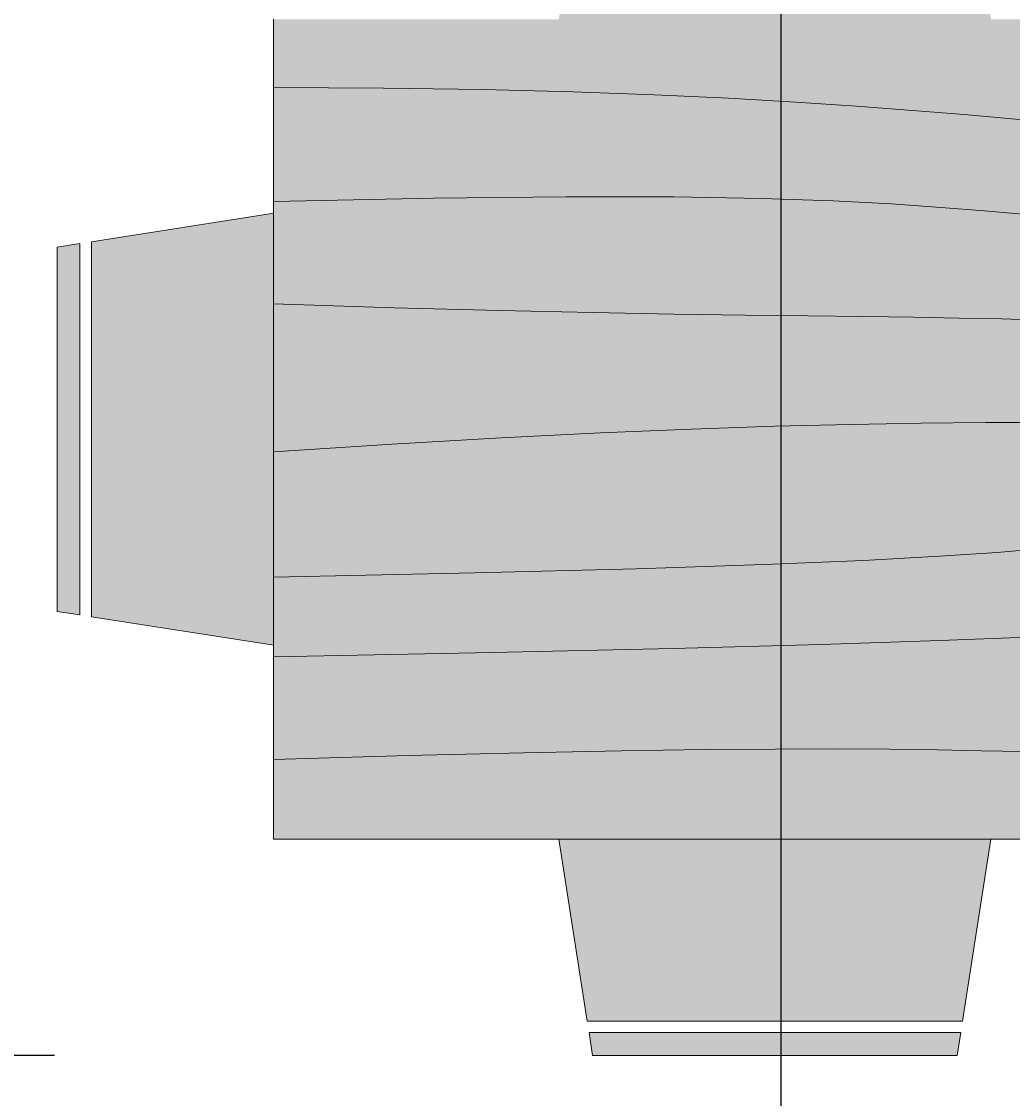
# Model space of a CAD drawing. Units: inches. Extents: x 2549 to 3108, y 1683 to 2362.
# Tile 9 of 30: x 2711 to 2734, y 2016 to 2041. Entities that reach past the tile are written whole.
import ezdxf

# ---------------------------------------------------------------- set-up
doc = ezdxf.new("R2010")
doc.units = ezdxf.units.IN
for name, color, linetype, lineweight in [('A-ANNO-DIMS', 2, 'Continuous', 18), ('A-FURN', 8, 'Continuous', 18), ('A-FURN-PATT', 9, 'Continuous', 13)]:
    doc.layers.add(name, color=color, linetype=linetype, lineweight=lineweight)
doc.layers.add('C-PKNG-VEHI-PATT', color=251, linetype='Continuous', lineweight=13, true_color=0x636466)
doc.layers.add('C-PVMT-PATT', color=9, linetype='Continuous', lineweight=13, true_color=0xc7c8ca)
doc.styles.get("Standard").update_dxf_attribs({"font": 'arial.ttf'})
doc.dimstyles.get("Standard").update_dxf_attribs({"dimtxt": 0.18, "dimasz": 0.18, "dimexe": 0.18, "dimexo": 0.0625, "dimgap": 0.09, "dimtad": 0, "dimtih": 1, "dimtoh": 1, "dimdec": 4, "dimzin": 0, "dimdsep": 46, "dimtxsty": 'Standard', "dimcen": 0.09, "dimadec": 0, "dimazin": 0, "dimtfac": 1, "dimtdec": 4, "dimtofl": 0, "dimtmove": 0, "dimatfit": 3, "dimfxl": 1, "dimtolj": 1, "dimtzin": 0, "dimarcsym": 0})

# ---------------------------------------------------------------- blocks, each defined once
blk = doc.blocks.new('Dining Set - 36 x 72 in.')
for p, q in [((-36, 18), (-36, -18)), ((-44.0006, 8.23428), (-35.9976, 9.48474)), ((-45.5, 8), (-44.5004, 8.15617)), ((-44.5, -8.15843), (-44.5, 8.15338)), ((-44, 8.23041), (-44, -8.23915)), ((-45.5, 8), (-45.5, -8)), ((-44.4997, -8.15631), (-45.5, -8)), ((-35.9976, -9.48476), (-43.9993, -8.2345)), ((-36, -18), (36, -18)), ((-22.2343, -26.0006), (-23.4847, -17.99762)), ((-4.5152, -17.99762), (-5.7655, -25.99928)), ((-22.2304, -26), (-5.7608, -26)), ((-22, -27.5), (-22.1562, -26.50044)), ((-5.8416, -26.5), (-22.1534, -26.5)), ((-5.8437, -26.49967), (-6, -27.5)), ((-22, -27.5), (-6, -27.5))]:
    blk.add_line(p, q)
for points in [[(-36, 15), (-31.1772, 14.97754), (-26.8079, 14.91406), (-22.8538, 14.81543), (-19.276, 14.6875), (-16.0362, 14.53613), (-13.0957, 14.36718), (-10.4159, 14.18652), (-7.9583, 14), (-5.6904, 13.81315), (-3.6035, 13.63021), (-1.6954, 13.45508)], [(-36, 10), (-28.9766, 10.14274), (-23.1725, 10.20442), (-18.4241, 10.19775), (-14.5677, 10.13541), (-11.4399, 10.03011), (-8.877, 9.89453), (-6.7154, 9.74137), (-4.7917, 9.58333), (-2.9698, 9.43082)], [(-36, 5.5), (-30.7157, 5.3348), (-26.069, 5.20963), (-21.9946, 5.11767), (-18.4271, 5.05208), (-15.3009, 5.00602), (-12.5508, 4.97265), (-10.1112, 4.94515), (-7.9167, 4.91666), (-5.909, 4.88167), (-4.0586, 4.83984), (-2.3429, 4.79215)], [(-36, -1), (-30.7915, -0.6591), (-26.0195, -0.38216), (-21.6519, -0.16284), (-17.6563, 0.00521), (-14.0005, 0.12833), (-10.6523, 0.21289), (-7.5796, 0.26522), (-4.75, 0.29166), (-2.134, 0.29793)], [(-36, -6.5), (-27.1843, -6.31267), (-20.084, -6.1263), (-14.469, -5.9419), (-10.1094, -5.76042), (-6.7752, -5.58285), (-4.2363, -5.41016), (-2.2629, -5.24333)], [(-36, -10), (-26.4022, -9.81299), (-18.4675, -9.62891), (-11.9839, -9.45069), (-6.7396, -9.28125), (-2.5226, -9.12354)], [(-36, -14.5), (-30.0881, -14.33513), (-25.0332, -14.21224), (-20.7312, -14.12647), (-17.0781, -14.07292), (-13.97, -14.04671), (-11.3027, -14.04297), (-8.9724, -14.05681), (-6.875, -14.08334), (-4.9224, -14.11833), (-3.0905, -14.16016)]]:
    blk.add_lwpolyline(points)
blk = doc.blocks.new('*D21')
at = {"layer": 'A-ANNO-DIMS', "color": 0, "lineweight": -2, "transparency": 16777216}
for p, q in [((2711.452, 2046.283), (2703.972, 2046.283)), ((2704.152, 2046.103), (2704.152, 2031.633)), ((2704.152, 2016.798), (2704.152, 2031.269)), ((2711.452, 2016.618), (2703.972, 2016.618))]:
    blk.add_line(p, q, dxfattribs=at)
at = {"layer": 'A-ANNO-DIMS', "color": 0, "transparency": 16777216}
for points in [[(2704.122, 2046.103), (2704.182, 2046.103), (2704.152, 2046.283)], [(2704.122, 2016.798), (2704.182, 2016.798), (2704.152, 2016.618)]]:
    blk.add_solid(points, dxfattribs=at)
at = {"layer": 'Defpoints', "color": 0, "transparency": 16777216}
for p in [(2704.152, 2046.283), (2711.514, 2046.283), (2711.514, 2016.618)]:
    blk.add_point(p, dxfattribs=at)
at = {"layer": 'A-ANNO-DIMS', "color": 0, "transparency": 16777216, "insert": (2704.152, 2031.451), "char_height": 0.18, "attachment_point": 5}
blk.add_mtext('\\A1;30', dxfattribs=at)
blk = doc.blocks.new('*D42')
at = {"layer": 'A-ANNO-DIMS', "color": 0, "lineweight": -2, "transparency": 16777216}
for p, q in [((2638.643, 2080.461), (2638.643, 1683.444)), ((2728.643, 2080.461), (2728.643, 1683.444)), ((2638.823, 1683.624), (2683.424, 1683.624)), ((2728.463, 1683.624), (2683.861, 1683.624))]:
    blk.add_line(p, q, dxfattribs=at)
at = {"layer": 'A-ANNO-DIMS', "color": 0, "transparency": 16777216}
for points in [[(2638.823, 1683.654), (2638.823, 1683.594), (2638.643, 1683.624)], [(2728.463, 1683.654), (2728.463, 1683.594), (2728.643, 1683.624)]]:
    blk.add_solid(points, dxfattribs=at)
at = {"layer": 'Defpoints', "color": 0, "transparency": 16777216}
for p in [(2638.643, 2080.524), (2728.643, 2080.524), (2728.643, 1683.624)]:
    blk.add_point(p, dxfattribs=at)
at = {"layer": 'A-ANNO-DIMS', "color": 0, "transparency": 16777216, "insert": (2683.643, 1683.624), "char_height": 0.18, "attachment_point": 5}
blk.add_mtext('\\A1;90', dxfattribs=at)
blk = doc.blocks.new('*D44')
at = {"layer": 'A-ANNO-DIMS', "color": 0, "lineweight": -2, "transparency": 16777216}
for p, q in [((2662.643, 2040.993), (2662.643, 1683.444)), ((2806.643, 2016.129), (2806.643, 1683.444)), ((2662.823, 1683.624), (2734.363, 1683.624)), ((2806.463, 1683.624), (2734.923, 1683.624))]:
    blk.add_line(p, q, dxfattribs=at)
at = {"layer": 'A-ANNO-DIMS', "color": 0, "transparency": 16777216}
for points in [[(2662.823, 1683.654), (2662.823, 1683.594), (2662.643, 1683.624)], [(2806.463, 1683.654), (2806.463, 1683.594), (2806.643, 1683.624)]]:
    blk.add_solid(points, dxfattribs=at)
at = {"layer": 'Defpoints', "color": 0, "transparency": 16777216}
for p in [(2662.643, 2041.056), (2806.643, 2016.191), (2806.643, 1683.624)]:
    blk.add_point(p, dxfattribs=at)
at = {"layer": 'A-ANNO-DIMS', "color": 0, "transparency": 16777216, "insert": (2734.643, 1683.624), "char_height": 0.18, "attachment_point": 5}
blk.add_mtext('\\A1;144', dxfattribs=at)
blk = doc.blocks.new('*D59')
at = {"layer": 'A-ANNO-DIMS', "color": 0, "lineweight": -2, "transparency": 16777216}
for p, q in [((2680.978, 1761.586), (2680.978, 2362.323)), ((2681.158, 2362.143), (2733.112, 2362.143)), ((2785.978, 2362.143), (2734.023, 2362.143)), ((2786.158, 1761.586), (2786.158, 2362.323))]:
    blk.add_line(p, q, dxfattribs=at)
at = {"layer": 'A-ANNO-DIMS', "color": 0, "transparency": 16777216}
for points in [[(2681.158, 2362.173), (2681.158, 2362.113), (2680.978, 2362.143)], [(2785.978, 2362.173), (2785.978, 2362.113), (2786.158, 2362.143)]]:
    blk.add_solid(points, dxfattribs=at)
at = {"layer": 'Defpoints', "color": 0, "transparency": 16777216}
for p in [(2786.158, 2362.143), (2680.978, 1761.524), (2786.158, 1761.524)]:
    blk.add_point(p, dxfattribs=at)
at = {"layer": 'A-ANNO-DIMS', "color": 0, "transparency": 16777216, "insert": (2733.568, 2362.143), "char_height": 0.18, "attachment_point": 5}
blk.add_mtext('\\A1;105.18', dxfattribs=at)

msp = doc.modelspace()

# ---------------------------------------------------------------- hatches: boundary and pattern name
at = {"layer": 'A-FURN-PATT'}
h = msp.add_hatch(color=256, dxfattribs=at)
h.dxf.hatch_style = 1
h.paths.add_polyline_path([(2732.9458, 2045.4744), (2724.0631, 2045.4744), (2723.389, 2041.1594), (2733.6201, 2041.1594)])
h.paths.add_polyline_path([(2748.0481, 2045.4744), (2739.1654, 2045.4744), (2738.4912, 2041.1594), (2748.7223, 2041.1594)])
h.paths.add_polyline_path([(2747.9217, 2046.2834), (2739.2918, 2046.2834), (2739.2075, 2045.7441), (2748.006, 2045.7441)])
h.paths.add_polyline_path([(2732.8194, 2046.2834), (2724.1896, 2046.2834), (2724.1053, 2045.7441), (2732.9037, 2045.7441)])
h.paths.add_polyline_path([(2759.7877, 2035.8922), (2755.4728, 2036.5664), (2755.4728, 2026.3353), (2759.7877, 2027.0095)])
h.paths.add_polyline_path([(2760.5968, 2035.7658), (2760.0574, 2035.8501), (2760.0574, 2027.0516), (2760.5968, 2027.1359)])
h.paths.add_polyline_path([(2716.6384, 2036.5664), (2712.3235, 2035.8922), (2712.3235, 2027.0095), (2716.6384, 2026.3353)])
h.paths.add_polyline_path([(2733.6201, 2021.7423), (2723.389, 2021.7423), (2724.0631, 2017.4273), (2732.9458, 2017.4273)])
h.paths.add_polyline_path([(2748.7223, 2021.7423), (2738.4912, 2021.7423), (2739.1654, 2017.4273), (2748.0481, 2017.4273)])
h.paths.add_polyline_path([(2748.006, 2017.1576), (2739.2075, 2017.1576), (2739.2918, 2016.6183), (2747.9217, 2016.6183)])
h.paths.add_polyline_path([(2732.9037, 2017.1576), (2724.1053, 2017.1576), (2724.1896, 2016.6183), (2732.8194, 2016.6183)])
h.paths.add_polyline_path([(2712.0538, 2035.85), (2711.5145, 2035.7658), (2711.5145, 2027.1359), (2712.0538, 2027.0516)])
h = msp.add_hatch(color=256, dxfattribs=at)
h.dxf.hatch_style = 1
h.paths.add_polyline_path([(2744.8667, 2037.254), (2744.7754, 2037.3839), (2744.7125, 2037.4849), (2744.6595, 2037.5854), (2744.5963, 2037.7375), (2744.5695, 2037.9287), (2744.6003, 2038.0617), (2744.6406, 2038.148), (2744.7014, 2038.2298), (2744.7817, 2038.3053), (2744.8799, 2038.3724), (2744.9945, 2038.4289), (2745.1238, 2038.4728), (2745.2663, 2038.5019), (2745.4204, 2038.5142), (2745.5844, 2038.5076), (2745.7585, 2038.4805), (2745.9486, 2038.4342), (2746.1624, 2038.3705), (2746.4075, 2038.2913), (2746.6917, 2038.1983), (2747.0224, 2038.0936), (2747.4074, 2037.9788), (2747.8543, 2037.8558), (2748.3724, 2037.7256), (2748.9783, 2037.5851), (2749.69, 2037.4304), (2750.5258, 2037.2575), (2751.5038, 2037.0624), (2752.6422, 2036.8414), (2753.9591, 2036.5902), (2755.4728, 2036.3051), (2755.4728, 2039.002), (2754.0892, 2039.103), (2752.7721, 2039.2035), (2751.5251, 2039.303), (2750.3516, 2039.4009), (2749.255, 2039.4967), (2748.2388, 2039.5898), (2747.3063, 2039.6798), (2746.4609, 2039.7661), (2745.7045, 2039.8482), (2745.0321, 2039.9255), (2744.4371, 2039.9976), (2743.9129, 2040.0639), (2743.4531, 2040.1238), (2743.0509, 2040.1769), (2742.6998, 2040.2227), (2742.3932, 2040.2605), (2742.1251, 2040.29), (2741.8917, 2040.3111), (2741.69, 2040.3237), (2741.5167, 2040.3279), (2741.3687, 2040.3237), (2741.2428, 2040.3111), (2741.1359, 2040.29), (2741.0448, 2040.2605), (2740.9668, 2040.2227), (2740.9015, 2040.1776), (2740.8488, 2040.1262), (2740.8088, 2040.0695), (2740.7814, 2040.0085), (2740.7667, 2039.9445), (2740.7646, 2039.8783), (2740.7751, 2039.811), (2740.7978, 2039.7435), (2740.8306, 2039.6755), (2740.8707, 2039.6064), (2740.9155, 2039.5357), (2740.996, 2039.4111), (2741.0771, 2039.2637), (2741.1346, 2039.0945), (2741.1499, 2038.9139), (2741.1092, 2038.7391), (2741.0289, 2038.6239), (2740.9549, 2038.5525), (2740.8586, 2038.4895), (2740.733, 2038.4359), (2740.5693, 2038.3929), (2740.3593, 2038.3615), (2740.0946, 2038.3427), (2739.7666, 2038.3376), (2739.367, 2038.3473), (2738.8873, 2038.3727), (2738.3203, 2038.4145), (2737.6635, 2038.471), (2736.9156, 2038.5402), (2736.0753, 2038.6199), (2735.1412, 2038.7081), (2734.112, 2038.8025), (2732.9864, 2038.9012), (2731.7632, 2039.002), (2730.4376, 2039.1026), (2728.9922, 2039.2), (2727.4062, 2039.2911), (2725.6588, 2039.3728), (2723.7291, 2039.4418), (2721.5964, 2039.495), (2719.2397, 2039.5292), (2716.6384, 2039.5413), (2716.6384, 2036.8445), (2720.4266, 2036.9215), (2723.5572, 2036.9548), (2726.1183, 2036.9512), (2728.1983, 2036.9175), (2729.8853, 2036.8608), (2731.2677, 2036.7876), (2732.4336, 2036.705), (2733.4711, 2036.6198), (2734.4538, 2036.5375), (2735.3951, 2036.4589), (2736.2938, 2036.3835), (2737.1484, 2036.3108), (2737.9578, 2036.2401), (2738.7205, 2036.171), (2739.4353, 2036.103), (2740.1009, 2036.0355), (2740.7163, 2035.9683), (2741.2828, 2035.9027), (2741.8019, 2035.8403), (2742.2752, 2035.7826), (2742.7042, 2035.7313), (2743.0906, 2035.6878), (2743.4358, 2035.6539), (2743.7416, 2035.6309), (2744.0097, 2035.6203), (2744.243, 2035.6218), (2744.4448, 2035.6349), (2744.6181, 2035.659), (2744.7661, 2035.6937), (2744.892, 2035.7384), (2744.9989, 2035.7926), (2745.09, 2035.8557), (2745.1679, 2035.9271), (2745.2326, 2036.006), (2745.2836, 2036.0911), (2745.3204, 2036.1815), (2745.3424, 2036.2762), (2745.3492, 2036.374), (2745.3401, 2036.4739), (2745.3148, 2036.5748), (2745.2731, 2036.676), (2745.2178, 2036.7771), (2745.152, 2036.8782), (2745.0788, 2036.9794), (2745.0013, 2037.0805)])
h.paths.add_polyline_path([(2755.4728, 2036.3051), (2753.9591, 2036.5902), (2752.6422, 2036.8414), (2751.5038, 2037.0624), (2750.5258, 2037.2575), (2749.69, 2037.4304), (2748.9783, 2037.5851), (2748.3724, 2037.7256), (2747.8543, 2037.8558), (2747.4074, 2037.9788), (2747.0224, 2038.0936), (2746.6917, 2038.1983), (2746.4075, 2038.2913), (2746.1624, 2038.3705), (2745.9486, 2038.4342), (2745.7585, 2038.4805), (2745.5844, 2038.5076), (2745.4204, 2038.5142), (2745.2663, 2038.5019), (2745.1238, 2038.4728), (2744.9945, 2038.4289), (2744.8799, 2038.3724), (2744.7817, 2038.3053), (2744.7014, 2038.2298), (2744.6406, 2038.148), (2744.6003, 2038.0617), (2744.5794, 2037.9717), (2744.5765, 2037.8786), (2744.59, 2037.7828), (2744.6182, 2037.6849), (2744.6595, 2037.5854), (2744.7125, 2037.4849), (2744.7754, 2037.3839), (2744.8465, 2037.2827), (2744.9229, 2037.1816), (2745.0013, 2037.0805), (2745.1278, 2036.9154), (2745.2178, 2036.7771), (2745.2731, 2036.676), (2745.3148, 2036.5748), (2745.3401, 2036.4739), (2745.3492, 2036.374), (2745.3424, 2036.2762), (2745.3204, 2036.1815), (2745.2836, 2036.0911), (2745.2326, 2036.006), (2745.1679, 2035.9271), (2745.09, 2035.8557), (2744.9989, 2035.7926), (2744.892, 2035.7384), (2744.7661, 2035.6937), (2744.6181, 2035.659), (2744.4448, 2035.6349), (2744.243, 2035.6218), (2744.0097, 2035.6203), (2743.7416, 2035.6309), (2743.4358, 2035.6539), (2743.0906, 2035.6878), (2742.7042, 2035.7313), (2742.2752, 2035.7826), (2741.8019, 2035.8403), (2741.2828, 2035.9027), (2740.7163, 2035.9683), (2740.1009, 2036.0355), (2739.4353, 2036.103), (2738.7205, 2036.171), (2737.9578, 2036.2401), (2737.1484, 2036.3108), (2736.2938, 2036.3835), (2735.3951, 2036.4589), (2734.4538, 2036.5375), (2733.4711, 2036.6198), (2732.4336, 2036.705), (2731.2677, 2036.7876), (2729.8853, 2036.8608), (2728.1983, 2036.9175), (2726.1183, 2036.9512), (2723.5572, 2036.9548), (2720.4266, 2036.9215), (2716.6384, 2036.8445), (2716.6384, 2034.4174), (2719.4886, 2034.3283), (2721.9949, 2034.2608), (2724.1925, 2034.2112), (2726.1167, 2034.1758), (2727.8028, 2034.1509), (2729.2861, 2034.1329), (2730.602, 2034.1181), (2731.7856, 2034.1027), (2732.8685, 2034.0839), (2733.8666, 2034.0613), (2734.7919, 2034.0356), (2735.6567, 2034.0072), (2736.473, 2033.9768), (2737.253, 2033.9447), (2738.0088, 2033.9116), (2738.7525, 2033.878), (2739.493, 2033.8445), (2740.2273, 2033.812), (2740.9489, 2033.7816), (2741.6515, 2033.7544), (2742.3289, 2033.7314), (2742.9747, 2033.7137), (2743.5825, 2033.7022), (2744.1461, 2033.6982), (2744.6607, 2033.7024), (2745.1272, 2033.7151), (2745.5485, 2033.7361), (2745.9272, 2033.7656), (2746.2658, 2033.8036), (2746.567, 2033.8499), (2746.8334, 2033.9047), (2747.0677, 2033.9679), (2747.2728, 2034.0393), (2747.4525, 2034.1175), (2747.6113, 2034.201), (2747.7531, 2034.2881), (2747.8824, 2034.3774), (2748.0032, 2034.4672), (2748.1197, 2034.556), (2748.2363, 2034.6421), (2748.3567, 2034.7241), (2748.4828, 2034.8008), (2748.6163, 2034.8712), (2748.7588, 2034.9343), (2748.9118, 2034.9889), (2749.077, 2035.034), (2749.2558, 2035.0686), (2749.4499, 2035.0916), (2749.6603, 2035.1022), (2749.8861, 2035.1007), (2750.1254, 2035.0876), (2750.3769, 2035.0635), (2750.639, 2035.0288), (2750.91, 2034.9841), (2751.1884, 2034.93), (2751.4725, 2034.8668), (2751.7642, 2034.7949), (2752.0786, 2034.7123), (2752.4341, 2034.6172), (2752.849, 2034.5073), (2753.3419, 2034.3805), (2753.9313, 2034.2348), (2754.6354, 2034.068), (2755.4728, 2033.878)])
h.paths.add_polyline_path([(2755.4728, 2033.878), (2754.6354, 2034.068), (2753.9313, 2034.2348), (2753.3419, 2034.3805), (2752.849, 2034.5073), (2752.4341, 2034.6172), (2752.0786, 2034.7123), (2751.7642, 2034.7949), (2751.4725, 2034.8668), (2751.1884, 2034.93), (2750.91, 2034.9841), (2750.639, 2035.0288), (2750.3769, 2035.0635), (2750.1254, 2035.0876), (2749.8861, 2035.1007), (2749.6603, 2035.1022), (2749.4499, 2035.0916), (2749.2558, 2035.0686), (2749.077, 2035.034), (2748.9118, 2034.9889), (2748.7588, 2034.9343), (2748.6163, 2034.8712), (2748.4828, 2034.8008), (2748.3567, 2034.7241), (2748.2363, 2034.6421), (2748.1197, 2034.556), (2748.0032, 2034.4672), (2747.8824, 2034.3774), (2747.7531, 2034.2881), (2747.6113, 2034.201), (2747.4525, 2034.1175), (2747.2728, 2034.0393), (2747.0677, 2033.9679), (2746.8334, 2033.9047), (2746.567, 2033.8499), (2746.2658, 2033.8036), (2745.9272, 2033.7656), (2745.5485, 2033.7361), (2745.1272, 2033.7151), (2744.6607, 2033.7024), (2744.1461, 2033.6982), (2743.5825, 2033.7022), (2742.9747, 2033.7137), (2742.3289, 2033.7314), (2741.6515, 2033.7544), (2740.9489, 2033.7816), (2740.2273, 2033.812), (2739.493, 2033.8445), (2738.7525, 2033.878), (2738.0088, 2033.9116), (2737.253, 2033.9447), (2736.473, 2033.9768), (2735.6567, 2034.0072), (2734.7919, 2034.0356), (2733.8666, 2034.0613), (2732.8685, 2034.0839), (2731.7856, 2034.1027), (2730.602, 2034.1181), (2729.2861, 2034.1329), (2727.8028, 2034.1509), (2726.1167, 2034.1758), (2724.1925, 2034.2112), (2721.9949, 2034.2608), (2719.4886, 2034.3283), (2716.6384, 2034.4174), (2716.6384, 2030.9115), (2719.4477, 2031.0954), (2722.0216, 2031.2447), (2724.3773, 2031.363), (2726.5324, 2031.4537), (2728.5042, 2031.5201), (2730.3101, 2031.5657), (2731.9674, 2031.5939), (2733.4936, 2031.6082), (2734.9046, 2031.6115), (2736.2109, 2031.6057), (2737.4211, 2031.592), (2738.5446, 2031.5716), (2739.59, 2031.5461), (2740.5665, 2031.5165), (2741.4829, 2031.4843), (2742.3482, 2031.4509), (2743.1698, 2031.4174), (2743.9488, 2031.3855), (2744.6845, 2031.3568), (2745.3766, 2031.3329), (2746.0244, 2031.3152), (2746.6274, 2031.3055), (2747.1851, 2031.3052), (2747.697, 2031.316), (2748.1634, 2031.3388), (2748.5882, 2031.3722), (2748.9761, 2031.414), (2749.3319, 2031.4621), (2749.6603, 2031.5144), (2749.9661, 2031.5688), (2750.254, 2031.6233), (2750.5287, 2031.6756), (2750.7946, 2031.7239), (2751.0553, 2031.7669), (2751.314, 2031.8036), (2751.5737, 2031.8329), (2751.8375, 2031.8538), (2752.1088, 2031.8652), (2752.3906, 2031.8661), (2752.6861, 2031.8554), (2752.9965, 2031.8326), (2753.315, 2031.7999), (2753.633, 2031.7598), (2753.9418, 2031.7149), (2754.2327, 2031.6679), (2754.497, 2031.6215), (2754.7259, 2031.5782), (2754.911, 2031.5407), (2755.0467, 2031.5111), (2755.141, 2031.4888), (2755.2053, 2031.4728), (2755.2509, 2031.4621), (2755.2891, 2031.4556), (2755.3313, 2031.4523), (2755.3888, 2031.451), (2755.4728, 2031.4509)])
h.paths.add_polyline_path([(2743.9488, 2031.3855), (2743.1698, 2031.4174), (2742.3482, 2031.4509), (2741.4829, 2031.4843), (2740.5665, 2031.5165), (2739.59, 2031.5461), (2738.5446, 2031.5716), (2737.4211, 2031.592), (2736.2109, 2031.6057), (2734.9046, 2031.6115), (2733.4936, 2031.6082), (2731.9674, 2031.5939), (2730.3101, 2031.5657), (2728.5042, 2031.5201), (2726.5324, 2031.4537), (2724.3773, 2031.363), (2722.0216, 2031.2447), (2719.4477, 2031.0954), (2716.6384, 2030.9115), (2716.6384, 2027.945), (2721.3933, 2028.046), (2725.223, 2028.1465), (2728.2515, 2028.246), (2730.603, 2028.3439), (2732.4013, 2028.4397), (2733.7707, 2028.5328), (2734.8351, 2028.6228), (2735.7185, 2028.7091), (2736.5253, 2028.7912), (2737.2808, 2028.8692), (2737.9904, 2028.9429), (2738.6597, 2029.0125), (2739.2943, 2029.0778), (2739.8997, 2029.1389), (2740.4813, 2029.1958), (2741.0448, 2029.2484), (2741.5952, 2029.2967), (2742.1361, 2029.3397), (2742.6708, 2029.3764), (2743.2022, 2029.4058), (2743.7337, 2029.4266), (2744.2683, 2029.4381), (2744.8093, 2029.4389), (2745.3597, 2029.4282), (2745.9213, 2029.4053), (2746.4897, 2029.3713), (2747.0592, 2029.3279), (2747.6239, 2029.2765), (2748.1781, 2029.2189), (2748.716, 2029.1564), (2749.2317, 2029.0909), (2749.7196, 2029.0237), (2750.1754, 2028.9563), (2750.602, 2028.8892), (2751.0039, 2028.8226), (2751.3854, 2028.7568), (2751.7512, 2028.6921), (2752.1057, 2028.6287), (2752.4532, 2028.5668), (2752.7985, 2028.5068), (2753.1447, 2028.4496), (2753.4913, 2028.399), (2753.8363, 2028.3595), (2754.1778, 2028.3355), (2754.514, 2028.3315), (2754.8432, 2028.352), (2755.1634, 2028.4014), (2755.4728, 2028.4843), (2755.4728, 2031.4509), (2755.3151, 2031.4512), (2755.2429, 2031.4634), (2755.141, 2031.4888), (2755.0467, 2031.5111), (2754.911, 2031.5407), (2754.7259, 2031.5782), (2754.497, 2031.6215), (2754.2327, 2031.6679), (2753.9418, 2031.7149), (2753.633, 2031.7598), (2753.315, 2031.7999), (2752.9965, 2031.8326), (2752.6861, 2031.8554), (2752.3906, 2031.8661), (2752.1088, 2031.8652), (2751.8375, 2031.8538), (2751.5737, 2031.8329), (2751.314, 2031.8036), (2751.0553, 2031.7669), (2750.7946, 2031.7239), (2750.5287, 2031.6756), (2750.254, 2031.6233), (2749.9661, 2031.5688), (2749.6603, 2031.5144), (2749.3319, 2031.4621), (2748.9761, 2031.414), (2748.5882, 2031.3722), (2748.1634, 2031.3388), (2747.697, 2031.316), (2747.1851, 2031.3052), (2746.6274, 2031.3055), (2746.0244, 2031.3152), (2745.3766, 2031.3329), (2744.6845, 2031.3568)])
h.paths.add_polyline_path([(2755.4728, 2028.4843), (2755.1634, 2028.4014), (2754.8432, 2028.352), (2754.514, 2028.3315), (2754.1778, 2028.3355), (2753.8363, 2028.3595), (2753.4913, 2028.399), (2753.1447, 2028.4496), (2752.7985, 2028.5068), (2752.4532, 2028.5668), (2752.1057, 2028.6287), (2751.7512, 2028.6921), (2751.3854, 2028.7568), (2751.0039, 2028.8226), (2750.602, 2028.8892), (2750.1754, 2028.9563), (2749.7196, 2029.0237), (2749.2317, 2029.0909), (2748.716, 2029.1564), (2748.1781, 2029.2189), (2747.6239, 2029.2765), (2747.0592, 2029.3279), (2746.4897, 2029.3713), (2745.9213, 2029.4053), (2745.3597, 2029.4282), (2744.8093, 2029.4389), (2744.2683, 2029.4381), (2743.7337, 2029.4266), (2743.2022, 2029.4058), (2742.6708, 2029.3764), (2742.1361, 2029.3397), (2741.5952, 2029.2967), (2741.0448, 2029.2484), (2740.4813, 2029.1958), (2739.8997, 2029.1389), (2739.2943, 2029.0778), (2738.6597, 2029.0125), (2737.9904, 2028.9429), (2737.2808, 2028.8692), (2736.5253, 2028.7912), (2735.7185, 2028.7091), (2734.8351, 2028.6228), (2733.7707, 2028.5328), (2732.4013, 2028.4397), (2730.603, 2028.3439), (2728.2515, 2028.246), (2725.223, 2028.1465), (2721.3933, 2028.046), (2716.6384, 2027.945), (2716.6384, 2023.63), (2719.8271, 2023.719), (2722.5536, 2023.7853), (2724.8739, 2023.8315), (2726.8443, 2023.8604), (2728.5207, 2023.8745), (2729.9593, 2023.8765), (2731.2162, 2023.8691), (2732.3475, 2023.8548), (2733.4006, 2023.8359), (2734.3887, 2023.8133), (2735.3162, 2023.7876), (2736.1877, 2023.7593), (2737.0074, 2023.7288), (2737.7801, 2023.6968), (2738.5101, 2023.6637), (2739.2019, 2023.63), (2739.8611, 2023.5965), (2740.4973, 2023.5644), (2741.1215, 2023.5348), (2741.7443, 2023.5092), (2742.3766, 2023.4889), (2743.0291, 2023.4752), (2743.7127, 2023.4693), (2744.4383, 2023.4727), (2745.2212, 2023.4875), (2746.096, 2023.5194), (2747.1021, 2023.575), (2748.2785, 2023.6609), (2749.6645, 2023.7837), (2751.2994, 2023.9499), (2753.2224, 2024.1662), (2755.4728, 2024.4391)])
h.paths.add_polyline_path([(2755.4728, 2026.3269), (2754.9554, 2026.3329), (2754.418, 2026.3497), (2753.8658, 2026.3755), (2753.3041, 2026.4083), (2752.7382, 2026.4465), (2752.1734, 2026.4881), (2751.6149, 2026.5312), (2751.068, 2026.5741), (2750.5357, 2026.6151), (2750.0124, 2026.6538), (2749.4902, 2026.6898), (2748.9611, 2026.723), (2748.4173, 2026.753), (2747.8508, 2026.7795), (2747.2537, 2026.8024), (2746.6182, 2026.8213), (2745.9367, 2026.8359), (2745.2024, 2026.8452), (2744.4091, 2026.8482), (2743.5505, 2026.8438), (2742.6204, 2026.8309), (2741.6122, 2026.8087), (2740.5198, 2026.7758), (2739.3368, 2026.7314), (2738.0388, 2026.6748), (2736.5297, 2026.6071), (2734.695, 2026.5299), (2732.4205, 2026.4449), (2729.5919, 2026.3535), (2726.0949, 2026.2573), (2721.8152, 2026.1581), (2716.6384, 2026.0572), (2716.6384, 2023.63), (2719.8271, 2023.719), (2722.5536, 2023.7853), (2724.8739, 2023.8315), (2726.8443, 2023.8604), (2728.5207, 2023.8745), (2729.9593, 2023.8765), (2731.2162, 2023.8691), (2732.3475, 2023.8548), (2733.4006, 2023.8359), (2734.3887, 2023.8133), (2735.3162, 2023.7876), (2736.1877, 2023.7593), (2737.0074, 2023.7288), (2737.7801, 2023.6968), (2738.5101, 2023.6637), (2739.2019, 2023.63), (2739.8611, 2023.5965), (2740.4973, 2023.5644), (2741.1215, 2023.5348), (2741.7443, 2023.5092), (2742.3766, 2023.4889), (2743.0291, 2023.4752), (2743.7127, 2023.4693), (2744.4383, 2023.4727), (2745.2212, 2023.4875), (2746.096, 2023.5194), (2747.1021, 2023.575), (2748.2785, 2023.6609), (2749.6645, 2023.7837), (2751.2994, 2023.9499), (2753.2224, 2024.1662), (2755.4728, 2024.4391)], flags=17)
h.paths.add_polyline_path([(2740.4973, 2023.5644), (2739.8611, 2023.5965), (2739.2019, 2023.63), (2738.5101, 2023.6637), (2737.7801, 2023.6968), (2737.0074, 2023.7288), (2736.1877, 2023.7593), (2735.3162, 2023.7876), (2734.3887, 2023.8133), (2733.4006, 2023.8359), (2732.3475, 2023.8548), (2731.2162, 2023.8691), (2729.9593, 2023.8765), (2728.5207, 2023.8745), (2726.8443, 2023.8604), (2724.8739, 2023.8315), (2722.5536, 2023.7853), (2719.8271, 2023.719), (2716.6384, 2023.63), (2716.6384, 2021.7423), (2755.4728, 2021.7423), (2755.4728, 2024.4391), (2753.2224, 2024.1662), (2751.2994, 2023.9499), (2749.6645, 2023.7837), (2748.2785, 2023.6609), (2747.1021, 2023.575), (2746.096, 2023.5194), (2745.2212, 2023.4875), (2744.4383, 2023.4727), (2743.7127, 2023.4693), (2743.0291, 2023.4752), (2742.3766, 2023.4889), (2741.7443, 2023.5092), (2741.1215, 2023.5348)])
h.paths.add_polyline_path([(2741.1359, 2040.29), (2741.2428, 2040.3111), (2741.3687, 2040.3237), (2741.5167, 2040.3279), (2741.69, 2040.3237), (2741.8917, 2040.3111), (2742.1251, 2040.29), (2742.3932, 2040.2605), (2742.6998, 2040.2227), (2743.0509, 2040.1769), (2743.4531, 2040.1238), (2743.9129, 2040.0639), (2744.4371, 2039.9976), (2745.0321, 2039.9255), (2745.7045, 2039.8482), (2746.4609, 2039.7661), (2747.3063, 2039.6798), (2748.2388, 2039.5898), (2749.255, 2039.4967), (2750.3516, 2039.4009), (2751.5251, 2039.303), (2752.7721, 2039.2035), (2754.0892, 2039.103), (2755.4728, 2039.002), (2755.4728, 2041.1594), (2716.6384, 2041.1594), (2716.6384, 2039.5413), (2719.2397, 2039.5292), (2721.5964, 2039.495), (2723.7291, 2039.4418), (2725.6588, 2039.3728), (2727.4062, 2039.2911), (2728.9922, 2039.2), (2730.4376, 2039.1026), (2731.7632, 2039.002), (2732.9864, 2038.9012), (2734.112, 2038.8025), (2735.1412, 2038.7081), (2736.0753, 2038.6199), (2736.9156, 2038.5402), (2737.6635, 2038.471), (2738.3203, 2038.4145), (2738.8873, 2038.3727), (2739.367, 2038.3473), (2739.7666, 2038.3376), (2740.0946, 2038.3427), (2740.3593, 2038.3615), (2740.5693, 2038.3929), (2740.733, 2038.4359), (2740.8586, 2038.4895), (2740.9549, 2038.5525), (2741.0289, 2038.6239), (2741.0834, 2038.7021), (2741.12, 2038.7856), (2741.1403, 2038.8728), (2741.1458, 2038.962), (2741.1382, 2039.0518), (2741.1189, 2039.1406), (2741.0897, 2039.2267), (2741.0522, 2039.309), (2741.0089, 2039.3875), (2740.9625, 2039.4629), (2740.8772, 2039.5951), (2740.8072, 2039.7159), (2740.7635, 2039.8453), (2740.7677, 2039.9782), (2740.8229, 2040.1009), (2740.9289, 2040.2044), (2741.0448, 2040.2605)])
h = msp.add_hatch(color=256, dxfattribs=at)
h.dxf.hatch_style = 1
h.paths.add_polyline_path([(2755.4728, 2026.3269), (2754.9554, 2026.3329), (2754.418, 2026.3497), (2753.8658, 2026.3755), (2753.3041, 2026.4083), (2752.7382, 2026.4465), (2752.1734, 2026.4881), (2751.6149, 2026.5312), (2751.068, 2026.5741), (2750.5357, 2026.6151), (2750.0124, 2026.6538), (2749.4902, 2026.6898), (2748.9611, 2026.723), (2748.4173, 2026.753), (2747.8508, 2026.7795), (2747.2537, 2026.8024), (2746.6182, 2026.8213), (2745.9367, 2026.8359), (2745.2024, 2026.8452), (2744.4091, 2026.8482), (2743.5505, 2026.8438), (2742.6204, 2026.8309), (2741.6122, 2026.8087), (2740.5198, 2026.7758), (2739.3368, 2026.7314), (2738.0388, 2026.6748), (2736.5297, 2026.6071), (2734.695, 2026.5299), (2732.4205, 2026.4449), (2729.5919, 2026.3535), (2726.0949, 2026.2573), (2721.8152, 2026.1581), (2716.6384, 2026.0572), (2716.6384, 2023.63), (2719.8271, 2023.719), (2722.5536, 2023.7853), (2724.8739, 2023.8315), (2726.8443, 2023.8604), (2728.5207, 2023.8745), (2729.9593, 2023.8765), (2731.2162, 2023.8691), (2732.3475, 2023.8548), (2733.4006, 2023.8359), (2734.3887, 2023.8133), (2735.3162, 2023.7876), (2736.1877, 2023.7593), (2737.0074, 2023.7288), (2737.7801, 2023.6968), (2738.5101, 2023.6637), (2739.2019, 2023.63), (2739.8611, 2023.5965), (2740.4973, 2023.5644), (2741.1215, 2023.5348), (2741.7443, 2023.5092), (2742.3766, 2023.4889), (2743.0291, 2023.4752), (2743.7127, 2023.4693), (2744.4383, 2023.4727), (2745.2212, 2023.4875), (2746.096, 2023.5194), (2747.1021, 2023.575), (2748.2785, 2023.6609), (2749.6645, 2023.7837), (2751.2994, 2023.9499), (2753.2224, 2024.1662), (2755.4728, 2024.4391)])
at = {"layer": 'C-PKNG-VEHI-PATT'}
h = msp.add_hatch(color=256, dxfattribs=at)
h.dxf.hatch_style = 1
edge = h.paths.add_edge_path()
edge.add_ellipse((2935.7258, 1791.964), major_axis=(-50.66, 0), ratio=0.8423039, start_angle=248.16505, end_angle=265.72258)
edge.add_line((2938.911, 1834.5507), (2925.8653, 1834.5507))
edge.add_ellipse((2929.0505, 1791.964), major_axis=(50.66, 0), ratio=0.8423039, start_angle=94.27742, end_angle=111.83495)
edge.add_line((2912.8508, 1832.3947), (2914.2044, 1822.2495))
edge.add_ellipse((2930.6538, 1783.1023), major_axis=(-49.3014, 0), ratio=0.8423039, start_angle=-85.12993, end_angle=-67.20809, ccw=False)
edge.add_line((2927.1247, 1824.5225), (2937.6516, 1824.5225))
edge.add_ellipse((2934.1225, 1783.1023), major_axis=(49.3014, 0), ratio=0.8423039, start_angle=67.20809, end_angle=85.12993, ccw=False)
edge.add_line((2950.5719, 1822.2495), (2951.9255, 1832.3947))
edge = h.paths.add_edge_path()
edge.add_ellipse((2903.4793, 1857.3351), major_axis=(-34.7979, 0), ratio=0.8423039, start_angle=180, end_angle=209.43857)
edge.add_ellipse((2961.297, 1857.3351), major_axis=(34.7979, 0), ratio=0.8423039, start_angle=150.56143, end_angle=180)
edge.add_line((2926.4991, 1857.3351), (2926.4991, 1843.7609))
edge.add_ellipse((2924.1251, 1844.3143), major_axis=(-0.2209, 3.9278), ratio=0.6038336, start_angle=89.00201, end_angle=253.65741, ccw=False)
edge.add_line((2921.7512, 1844.2222), (2921.7512, 1853.3975))
edge.add_line((2921.7512, 1853.3975), (2925.269, 1855.8484))
edge.add_ellipse((2925.4782, 1855.4931), major_axis=(0.4584, 0), ratio=0.8423039, start_angle=90, end_angle=134.48021, ccw=False)
edge.add_line((2925.4782, 1855.8792), (2926.4991, 1855.8792))
edge.add_line((2926.4991, 1855.8792), (2926.4991, 1857.3351))
edge.add_ellipse((2961.297, 1857.3351), major_axis=(34.7979, 0), ratio=0.8423039, start_angle=150.56143, end_angle=180, ccw=False)
edge.add_line((2932.3882, 1873.6501), (2932.3882, 1875.7801))
edge.add_ellipse((2932.3882, 1875.3939), major_axis=(0.4584, 0), ratio=0.8423039, start_angle=90, end_angle=127.93313)
edge.add_line((2932.1366, 1875.7167), (2928.5915, 1873.7564))
edge.add_ellipse((2899.9271, 2002.4692), major_axis=(155.4756, 0), ratio=0.84230387, start_angle=-80.743434, end_angle=-77.445067, ccw=False)
edge.add_ellipse((2949.4402, 1715.2151), major_axis=(-189.1422, 0), ratio=0.84230387, start_angle=-79.790461, end_angle=-77.555373)
edge.add_ellipse((3300.3614, 1852.5642), major_axis=(-386.1662, 0), ratio=0.84230387, start_angle=-2.863715, end_angle=2.198541)
edge.add_ellipse((2929.0505, 1792.5159), major_axis=(-55.6192, 0), ratio=0.8423039, start_angle=-85.91759, end_angle=-72.28005, ccw=False)
edge.add_line((2925.7129, 1839.2798), (2939.0634, 1839.2798))
edge.add_ellipse((2935.7258, 1792.5159), major_axis=(55.6192, 0), ratio=0.8423039, start_angle=72.28005, end_angle=85.91759, ccw=False)
edge.add_ellipse((2564.4149, 1852.5642), major_axis=(-386.1662, 0), ratio=0.84230387, start_angle=177.801459, end_angle=182.863715)
edge.add_ellipse((2915.3361, 1715.2151), major_axis=(189.1422, 0), ratio=0.84230387, start_angle=77.555373, end_angle=79.790461)
edge.add_ellipse((2964.8492, 2002.4692), major_axis=(-155.4756, 0), ratio=0.84230387, start_angle=77.445067, end_angle=80.743434, ccw=False)
edge.add_line((2936.1848, 1873.7564), (2932.6397, 1875.7167))
edge.add_ellipse((2932.3882, 1875.3939), major_axis=(0.4584, 0), ratio=0.8423039, start_angle=52.06687, end_angle=90)
edge.add_line((2932.3882, 1875.7801), (2932.3882, 1873.6501))
edge.add_ellipse((2903.4793, 1857.3351), major_axis=(-34.7979, 0), ratio=0.8423039, start_angle=180, end_angle=209.43857, ccw=False)
edge.add_line((2938.2772, 1857.3351), (2938.2772, 1855.8792))
edge.add_line((2938.2772, 1855.8792), (2939.4059, 1855.8792))
edge.add_ellipse((2939.2981, 1855.4931), major_axis=(-0.4584, 0), ratio=0.8423039, start_angle=225.51979, end_angle=270, ccw=False)
edge.add_line((2939.5903, 1855.7906), (2943.0251, 1853.3975))
edge.add_line((2943.0251, 1853.3975), (2943.0251, 1844.2222))
edge.add_ellipse((2940.6512, 1844.3143), major_axis=(0.2209, 3.9278), ratio=0.6038336, start_angle=106.34259, end_angle=270.99799, ccw=False)
edge.add_line((2938.2772, 1843.7609), (2938.2772, 1857.3351))
edge = h.paths.add_edge_path()
edge.add_ellipse((2932.3882, 1865.1973), major_axis=(91.081, 0), ratio=0.8423039, start_angle=256.401865, end_angle=283.598135, ccw=False)
edge.add_line((2914.2044, 1790.0239), (2914.2044, 1778.3622))
edge.add_ellipse((2932.3882, 1853.5356), major_axis=(91.081, 0), ratio=0.8423039, start_angle=256.401865, end_angle=283.598135)
edge.add_line((2950.5719, 1778.3622), (2950.5719, 1790.0239))
edge = h.paths.add_edge_path()
edge.add_ellipse((2948.7383, 1772.3145), major_axis=(1.8336, 0), ratio=0.8423039, start_angle=0, end_angle=90)
edge.add_line((2948.7383, 1773.859), (2916.038, 1773.859))
edge.add_ellipse((2916.038, 1772.3145), major_axis=(1.8336, 0), ratio=0.8423039, start_angle=90, end_angle=180)
edge.add_line((2914.2044, 1772.3145), (2914.2044, 1760.2558))
edge.add_line((2914.2044, 1760.2558), (2950.5719, 1760.2558))
edge.add_line((2950.5719, 1760.2558), (2950.5719, 1772.3145))
h.paths.add_polyline_path([(2748.8496, 2101.6383), (2798.148, 2101.6383), (2798.148, 2111.4248), (2748.8496, 2111.4248)], flags=9)
h.paths.add_polyline_path([(2685.2081, 2101.489), (2719.3253, 2101.489), (2719.3253, 2111.2819), (2685.2081, 2111.2819)], flags=9)
h.paths.add_polyline_path([(2814.6852, 1907.1328), (2847.8384, 1907.1328), (2847.8384, 1916.9258), (2814.6852, 1916.9258)], flags=9)
h.paths.add_polyline_path([(2814.3906, 1835.5864), (2848.0172, 1835.5864), (2848.0172, 1845.3794), (2814.3906, 1845.3794)], flags=9)
h.paths.add_polyline_path([(2800.5245, 1759.1674), (2853.7435, 1759.1674), (2853.7435, 1768.954), (2800.5245, 1768.954)], flags=9)
h.paths.add_polyline_path([(2972.4611, 1807.3305), (3015.3943, 1807.3305), (3015.3943, 1817.117), (2972.4611, 1817.117)], flags=9)
h.paths.add_polyline_path([(2902.3327, 1888.6731), (2937.9131, 1888.6731), (2937.9131, 1898.4661), (2902.3327, 1898.4661)], flags=9)
h.paths.add_polyline_path([(2712.1779, 1878.9039), (2754.1257, 1878.9039), (2754.1257, 1888.6904), (2712.1779, 1888.6904)], flags=9)
h.paths.add_polyline_path([(2614.0056, 2012.812), (2650.0251, 2012.812), (2650.0251, 2022.4371), (2614.0056, 2022.4371)], flags=9)
h.paths.add_polyline_path([(2713.3129, 2003.1645), (2747.4237, 2003.1645), (2747.4237, 2012.951), (2713.3129, 2012.951)], flags=9)
h.paths.add_polyline_path([(2950.1379, 2001.6934), (2982.2992, 2001.6934), (2982.2992, 2011.48), (2950.1379, 2011.48)], flags=9)
h.paths.add_polyline_path([(2940.864, 2238.5537), (2997.5066, 2238.5537), (2997.5066, 2248.3466), (2940.864, 2248.3466)], flags=9)
h.paths.add_polyline_path([(2821.5457, 2202.8348), (2855.663, 2202.8348), (2855.663, 2212.6278), (2821.5457, 2212.6278)], flags=9)
h.paths.add_polyline_path([(2661.8026, 2238.6249), (2718.4451, 2238.6249), (2718.4451, 2248.4179), (2661.8026, 2248.4179)], flags=9)
at = {"layer": 'C-PVMT-PATT'}
h = msp.add_hatch(color=256, dxfattribs=at)
h.dxf.hatch_style = 1
h.paths.add_polyline_path([(3067.6427, 2305.5237), (2605.6427, 2305.5237), (2605.6427, 2074.5237), (2629.6427, 2074.5237), (2629.6427, 2281.5237), (3043.6427, 2281.5237), (3043.6427, 1885.5237), (3043.6427, 1872.8745), (3031.1672, 1872.8745), (3031.1672, 1862.5731), (2995.8054, 1862.5731), (2995.8054, 1872.8745), (2983.1752, 1872.8745), (2983.1752, 1885.5237), (2881.6427, 1885.5237), (2881.6427, 1795.5237), (2751.0977, 1795.5237), (2751.0977, 1761.5237), (2786.1577, 1761.5237), (2786.1577, 1723.5237), (2881.84, 1723.5237), (2881.84, 1714.5237), (3067.6427, 1714.5237), (3067.6427, 1723.5237)])
edge = h.paths.add_edge_path(flags=16)
edge.add_ellipse((2949.4402, 1710.9683), major_axis=(-194.1014, 0), ratio=0.84230387, start_angle=-77.874034, end_angle=-76.219471, ccw=False)
edge.add_ellipse((2949.4402, 1715.2151), major_axis=(-189.1422, 0), ratio=0.84230387, start_angle=-79.790461, end_angle=-77.555373, ccw=False)
edge.add_ellipse((2899.9271, 2002.4692), major_axis=(155.4756, 0), ratio=0.84230387, start_angle=-80.743434, end_angle=-77.445067)
edge.add_line((2928.5915, 1873.7564), (2932.3882, 1875.8558))
edge.add_line((2932.3882, 1875.8558), (2936.1848, 1873.7564))
edge.add_ellipse((2964.8492, 2002.4692), major_axis=(-155.4756, 0), ratio=0.84230387, start_angle=77.445067, end_angle=80.743434)
edge.add_ellipse((2915.3361, 1715.2151), major_axis=(189.1422, 0), ratio=0.84230387, start_angle=77.555373, end_angle=79.790461, ccw=False)
edge.add_ellipse((2915.3361, 1710.9683), major_axis=(-194.1014, 0), ratio=0.84230387, start_angle=256.219471, end_angle=257.874034, ccw=False)
edge.add_ellipse((2628.2871, 1850.2612), major_axis=(-327.2532, 0), ratio=0.84230387, start_angle=182.17995, end_angle=183.650428, ccw=False)
edge.add_ellipse((2955.5637, 1861.9334), major_axis=(-0.9168, 0), ratio=0.8423039, start_angle=180, end_angle=270, ccw=False)
edge.add_line((2956.4805, 1862.3857), (2956.4805, 1846.4866))
edge.add_ellipse((2955.5637, 1846.939), major_axis=(-0.9168, 0), ratio=0.8423039, start_angle=90, end_angle=180, ccw=False)
edge.add_ellipse((-3607.0606, 1835.832), major_axis=(-6562.6242, 0), ratio=0.84230387, start_angle=179.61613322, end_angle=180.09022909, ccw=False)
edge.add_ellipse((2955.5637, 1791.0926), major_axis=(0.9168, 0), ratio=0.8423039, start_angle=0, end_angle=90, ccw=False)
edge.add_line((2956.4805, 1791.545), (2956.4805, 1775.6459))
edge.add_ellipse((2955.5637, 1776.0982), major_axis=(0.9168, 0), ratio=0.8423039, start_angle=270, end_angle=360, ccw=False)
edge.add_ellipse((-3607.0606, 1835.832), major_axis=(-6562.6242, 0), ratio=0.84230387, start_angle=179.3813568, end_angle=179.47172853, ccw=False)
edge.add_ellipse((2954.5907, 1763.8768), major_axis=(-1.3752, 0), ratio=0.8423039, start_angle=179.37176, end_angle=248.46476, ccw=False)
edge.add_ellipse((-3607.519, 1835.832), major_axis=(-6564.0409, 0), ratio=0.842303863, start_angle=179.35344594, end_angle=179.37176282, ccw=False)
edge.add_ellipse((2952.6829, 1761.8002), major_axis=(3.2503, 0), ratio=0.8423039, start_angle=-90, end_angle=-0.64655, ccw=False)
edge.add_line((2952.6829, 1759.0625), (2912.0934, 1759.0625))
edge.add_ellipse((2912.0934, 1761.8002), major_axis=(3.2503, 0), ratio=0.8423039, start_angle=180.64655, end_angle=270, ccw=False)
edge.add_ellipse((9472.2953, 1835.832), major_axis=(-6564.0409, 0), ratio=0.842303871, start_angle=0.62823722, end_angle=0.6465541, ccw=False)
edge.add_ellipse((2910.1856, 1763.8768), major_axis=(1.3752, 0), ratio=0.8423039, start_angle=111.53524, end_angle=180.62824, ccw=False)
edge.add_ellipse((9471.8369, 1835.832), major_axis=(-6562.6242, 0), ratio=0.84230387, start_angle=0.52827147, end_angle=0.6465541, ccw=False)
edge.add_ellipse((2909.2126, 1776.0982), major_axis=(-0.9168, 0), ratio=0.8423039, start_angle=0, end_angle=90, ccw=False)
edge.add_line((2908.2958, 1775.6459), (2908.2958, 1791.545))
edge.add_ellipse((2909.2126, 1791.0926), major_axis=(-0.9168, 0), ratio=0.8423039, start_angle=-90, end_angle=0, ccw=False)
edge.add_ellipse((9471.8369, 1835.832), major_axis=(-6562.6242, 0), ratio=0.84230387, start_angle=-0.09022909, end_angle=0.38386678, ccw=False)
edge.add_ellipse((2909.2126, 1846.939), major_axis=(-0.9168, 0), ratio=0.8423039, start_angle=0, end_angle=90, ccw=False)
edge.add_line((2908.2958, 1846.4866), (2908.2958, 1862.3857))
edge.add_ellipse((2909.2126, 1861.9334), major_axis=(0.9168, 0), ratio=0.8423039, start_angle=90, end_angle=180, ccw=False)
edge.add_ellipse((3236.4892, 1850.2612), major_axis=(327.2532, 0), ratio=0.84230387, start_angle=176.349572, end_angle=177.82005, ccw=False)
edge = h.paths.add_edge_path(flags=0)
edge.add_ellipse((2903.4793, 1857.3351), major_axis=(-34.7979, 0), ratio=0.8423039, start_angle=180, end_angle=209.43857, ccw=False)
edge.add_line((2938.2772, 1857.3351), (2938.2772, 1855.8792))
edge.add_line((2938.2772, 1855.8792), (2939.4631, 1855.8792))
edge.add_line((2939.4631, 1855.8792), (2943.0251, 1853.3975))
edge.add_line((2943.0251, 1853.3975), (2943.0251, 1844.2222))
edge.add_ellipse((2940.6512, 1844.3143), major_axis=(0.2209, 3.9278), ratio=0.6038336, start_angle=106.34259, end_angle=270.99799, ccw=False)
edge.add_line((2938.2772, 1843.7609), (2938.2772, 1857.3351))
edge.add_ellipse((2903.4793, 1857.3351), major_axis=(-34.7979, 0), ratio=0.8423039, start_angle=180, end_angle=209.43857)
edge.add_ellipse((2961.297, 1857.3351), major_axis=(34.7979, 0), ratio=0.8423039, start_angle=150.56143, end_angle=180)
edge.add_line((2926.4991, 1857.3351), (2926.4991, 1843.7609))
edge.add_ellipse((2924.1251, 1844.3143), major_axis=(-0.2209, 3.9278), ratio=0.6038336, start_angle=89.00201, end_angle=253.65741, ccw=False)
edge.add_line((2921.7512, 1844.2222), (2921.7512, 1853.3975))
edge.add_line((2921.7512, 1853.3975), (2925.3132, 1855.8792))
edge.add_line((2925.3132, 1855.8792), (2926.4991, 1855.8792))
edge.add_line((2926.4991, 1855.8792), (2926.4991, 1857.3351))
edge.add_ellipse((2961.297, 1857.3351), major_axis=(34.7979, 0), ratio=0.8423039, start_angle=150.56143, end_angle=180, ccw=False)
edge = h.paths.add_edge_path(flags=0)
edge.add_ellipse((2929.0505, 1791.964), major_axis=(50.66, 0), ratio=0.8423039, start_angle=94.27742, end_angle=111.83495, ccw=False)
edge.add_line((2925.8653, 1834.5507), (2938.911, 1834.5507))
edge.add_ellipse((2935.7258, 1791.964), major_axis=(-50.66, 0), ratio=0.8423039, start_angle=248.16505, end_angle=265.72258, ccw=False)
edge.add_line((2951.9255, 1832.3947), (2950.5719, 1822.2495))
edge.add_ellipse((2934.1225, 1783.1023), major_axis=(49.3014, 0), ratio=0.8423039, start_angle=67.20809, end_angle=85.12993)
edge.add_line((2937.6516, 1824.5225), (2927.1247, 1824.5225))
edge.add_ellipse((2930.6538, 1783.1023), major_axis=(-49.3014, 0), ratio=0.8423039, start_angle=-85.12993, end_angle=-67.20809)
edge.add_line((2914.2044, 1822.2495), (2912.8508, 1832.3947))
edge = h.paths.add_edge_path(flags=0)
edge.add_line((2910.1338, 1829.4651), (2912.6432, 1821.2711))
edge.add_ellipse((5203.7787, 1816.4367), major_axis=(-2291.1426, 0), ratio=0.84230387, start_angle=-0.1208974, end_angle=0.3640763)
edge.add_line((2912.7012, 1801.8782), (2910.3305, 1792.5698))
edge.add_ellipse((9471.8369, 1835.832), major_axis=(-6561.7074, 0), ratio=0.84230387, start_angle=0.05559431, end_angle=0.37776419, ccw=False)
edge = h.paths.add_edge_path(flags=0)
edge.add_ellipse((-3607.0606, 1835.832), major_axis=(6561.7074, 0), ratio=0.84230387, start_angle=-0.37776419, end_angle=-0.05559431, ccw=False)
edge.add_line((2954.4458, 1792.5698), (2952.0751, 1801.8782))
edge.add_ellipse((660.9976, 1816.4367), major_axis=(2291.1426, 0), ratio=0.84230387, start_angle=-0.3640763, end_angle=0.1208974)
edge.add_line((2952.1331, 1821.2711), (2954.6425, 1829.4651))
edge = h.paths.add_edge_path(flags=0)
edge.add_ellipse((2932.3882, 1865.1973), major_axis=(91.081, 0), ratio=0.8423039, start_angle=256.401865, end_angle=283.598135)
edge.add_line((2950.5719, 1790.0239), (2950.5719, 1778.3622))
edge.add_ellipse((2932.3882, 1853.5356), major_axis=(91.081, 0), ratio=0.8423039, start_angle=256.401865, end_angle=283.598135, ccw=False)
edge.add_line((2914.2044, 1778.3622), (2914.2044, 1790.0239))
edge = h.paths.add_edge_path(flags=0)
edge.add_line((2916.038, 1773.859), (2948.7383, 1773.859))
edge.add_ellipse((2948.7383, 1772.3145), major_axis=(1.8336, 0), ratio=0.8423039, start_angle=0, end_angle=90, ccw=False)
edge.add_line((2950.5719, 1772.3145), (2950.5719, 1760.2558))
edge.add_line((2950.5719, 1760.2558), (2914.2044, 1760.2558))
edge.add_line((2914.2044, 1760.2558), (2914.2044, 1772.3145))
edge.add_ellipse((2916.038, 1772.3145), major_axis=(1.8336, 0), ratio=0.8423039, start_angle=90, end_angle=180, ccw=False)
h.paths.add_polyline_path([(2629.6427, 1978.5237), (2605.6427, 1978.5237), (2605.6427, 1723.5237), (2629.6427, 1723.5237), (2629.6427, 1795.5237)], flags=17)
h.paths.add_polyline_path([(2800.5245, 1759.1674), (2853.7435, 1759.1674), (2853.7435, 1768.954), (2800.5245, 1768.954)], flags=24)
h.paths.add_polyline_path([(2972.4611, 1807.3305), (3015.3943, 1807.3305), (3015.3943, 1817.117), (2972.4611, 1817.117)], flags=24)

# ---------------------------------------------------------------- block references
at = {"layer": 'A-FURN', "xscale": 0.5393661791637867, "yscale": 0.5393661791637867, "zscale": 0.5393661791637867}
msp.add_blockref('Dining Set - 36 x 72 in.', (2736.0556, 2031.4509), dxfattribs=at)

# ---------------------------------------------------------------- dimensions: what is measured, and where the dimension line sits
at = {"layer": 'A-ANNO-DIMS'}
for base, p1, p2, override, picture, middle in [((2786.1577, 2362.1425), (2680.9778, 1761.5237), (2786.1577, 1761.5237), {"dimdec": 2, "dimlfac": 1, "dimrnd": 0, "dimzin": 0, "dimdsep": 46, "dimlunit": 2}, '*D59', (2733.5678, 2362.1425)), ((2728.6427, 1683.6237), (2638.6427, 2080.5237), (2728.6427, 2080.5237), {"dimdec": 0, "dimlfac": 1, "dimrnd": 0, "dimzin": 0, "dimdsep": 46, "dimlunit": 2}, '*D42', (2683.6427, 1683.6237)), ((2806.6427, 1683.6237), (2662.6427, 2041.0557), (2806.6427, 2016.1911), {"dimdec": 0, "dimlfac": 1, "dimrnd": 0, "dimzin": 0, "dimdsep": 46, "dimlunit": 2}, '*D44', (2734.6427, 1683.6237))]:
    dim = msp.add_linear_dim(base=base, p1=p1, p2=p2, dimstyle='Standard', override=override, dxfattribs=at)
    dim.commit()
    dim.dimension.update_dxf_attribs({"geometry": picture, "text_midpoint": middle})
dim = msp.add_linear_dim(base=(2704.1521, 2046.2834), p1=(2711.5145, 2016.6183), p2=(2711.5145, 2046.2834), angle=90, dimstyle='Standard', override={"dimdec": 0, "dimlfac": 1, "dimrnd": 0, "dimzin": 0, "dimdsep": 46, "dimlunit": 2}, dxfattribs=at)
dim.commit()
dim.dimension.update_dxf_attribs({"geometry": '*D21', "text_midpoint": (2704.1521, 2031.4509)})

doc.saveas('drawing.dxf')
